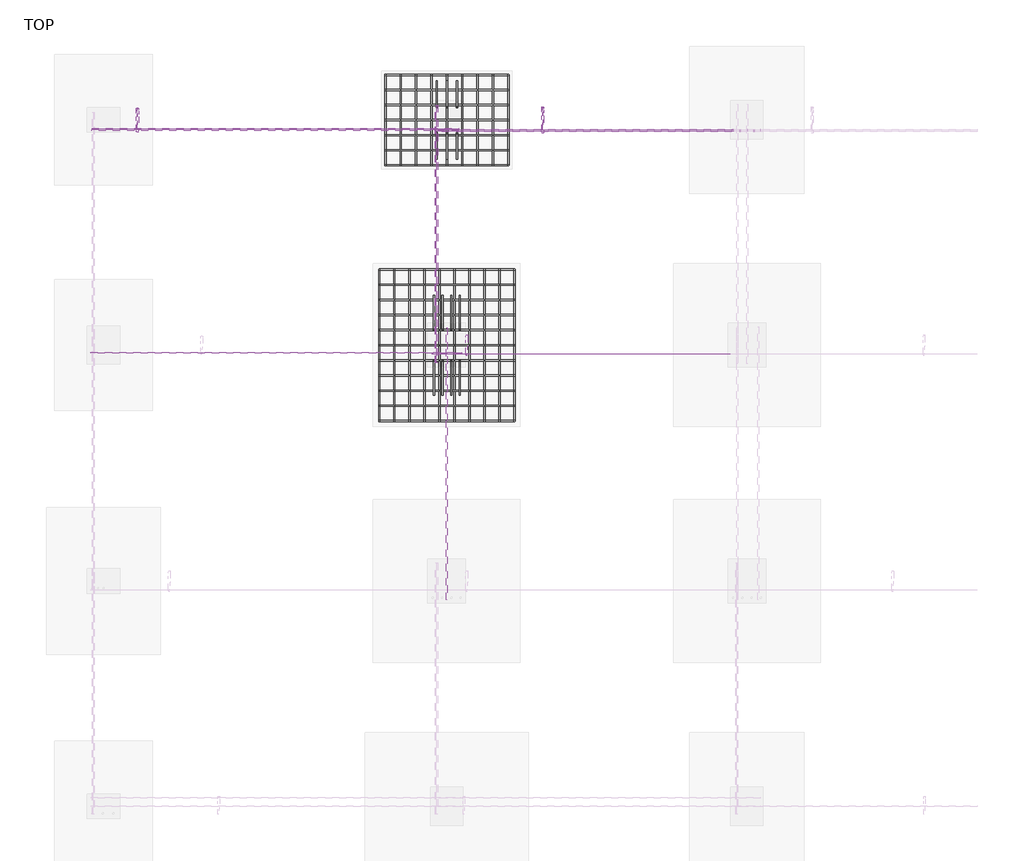
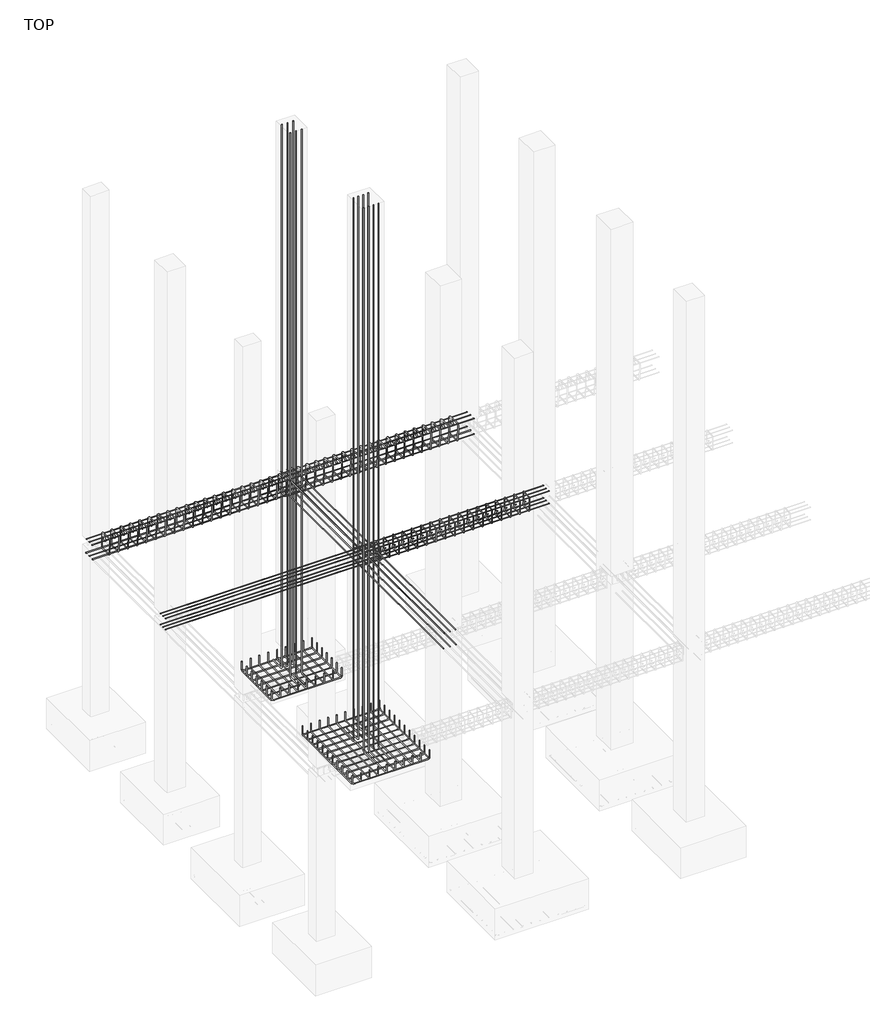
# One storey, part 4 of 8: 23 reinforcing bars.
"""IFC4 building model written with IfcOpenShell, lengths in millimetres."""

from ifc_helpers import new_model, si_unit, point, frame, origin, place, context, project, spatial, polyline, circle_curve, trimmed, segment, composite_curve, source, transform, mapped, element, save
from ifc_brep_helpers import swept_disk

model = new_model("IFC4")

# Units and contexts
model_context = context("Model", 3, world=origin())
ifc_project = project(units=[si_unit("LENGTHUNIT", "METRE", prefix="MILLI")], contexts=[model_context])

# Site, building, storey
site = spatial("IfcSite", under=ifc_project)
building = spatial("IfcBuilding", under=site)
storey = spatial("IfcBuildingStorey", under=building, Name="TOP", Elevation=0.0)

# Reinforcing bars
placement = place(None, origin())
reinforcing_bar_shape = source(origin(), model_context, "Body", "SolidModel", [
    swept_disk(composite_curve([segment(polyline([(-2538.5160601, 7943.1307576, -331.0), (-2538.5160601, 7943.1307576, -467.4)]), True, "CONTINUOUS"), segment(trimmed(circle_curve(frame((-2508.5160601, 7943.1307576, -467.4), z_axis=(0.0, -1.0, 0.0), x_axis=(-30.0, 0.0, 0.0)), 30.0), [point((-2538.5160601, 7943.1307576, -467.4))], [point((-2508.5160601, 7943.1307576, -497.4))], True, "CARTESIAN"), True, "CONTINUOUS"), segment(polyline([(-2508.5160601, 7943.1307576, -497.4), (-1421.3160601, 7943.1307576, -497.4)]), True, "CONTINUOUS"), segment(trimmed(circle_curve(frame((-1421.3160601, 7943.1307576, -467.4), z_axis=(0.0, -1.0, 0.0), x_axis=(0.0, 0.0, -30.0)), 30.0), [point((-1421.3160601, 7943.1307576, -497.4))], [point((-1391.3160601, 7943.1307576, -467.4))], True, "CARTESIAN"), True, "CONTINUOUS"), segment(polyline([(-1391.3160601, 7943.1307576, -467.4), (-1391.3160601, 7943.1307576, -331.0)]), True, "CONTINUOUS")], self_intersect=False), 6.0),
])
element("IfcReinforcingBar", 1, at=placement, inside=storey, context=model_context, shape_type="MappedRepresentation", body=[
    mapped(reinforcing_bar_shape, transform((0.0, 0.0, 0.0), x_axis=(1.0, 0.0, 0.0), y_axis=(0.0, 1.0, 0.0), z_axis=(0.0, 0.0, 1.0))),
    mapped(reinforcing_bar_shape, transform((0.0, -140.4, 0.0), x_axis=(1.0, 0.0, 0.0), y_axis=(0.0, 1.0, 0.0), z_axis=(0.0, 0.0, 1.0))),
    mapped(reinforcing_bar_shape, transform((0.0, -280.8, 0.0), x_axis=(1.0, 0.0, 0.0), y_axis=(0.0, 1.0, 0.0), z_axis=(0.0, 0.0, 1.0))),
    mapped(reinforcing_bar_shape, transform((0.0, -421.2, 0.0), x_axis=(1.0, 0.0, 0.0), y_axis=(0.0, 1.0, 0.0), z_axis=(0.0, 0.0, 1.0))),
    mapped(reinforcing_bar_shape, transform((0.0, -561.6, 0.0), x_axis=(1.0, 0.0, 0.0), y_axis=(0.0, 1.0, 0.0), z_axis=(0.0, 0.0, 1.0))),
    mapped(reinforcing_bar_shape, transform((0.0, -702.0, 0.0), x_axis=(1.0, 0.0, 0.0), y_axis=(0.0, 1.0, 0.0), z_axis=(0.0, 0.0, 1.0))),
    mapped(reinforcing_bar_shape, transform((0.0, -842.4, 0.0), x_axis=(1.0, 0.0, 0.0), y_axis=(0.0, 1.0, 0.0), z_axis=(0.0, 0.0, 1.0))),
])
reinforcing_bar_2_shape = source(origin(), model_context, "Body", "SolidModel", [
    swept_disk(composite_curve([segment(polyline([(-2538.5160601, 7100.7307576, -331.0), (-2538.5160601, 7100.7307576, -467.4)]), True, "CONTINUOUS"), segment(trimmed(circle_curve(frame((-2538.5160601, 7130.7307576, -467.4), z_axis=(1.0, 0.0, 0.0), x_axis=(0.0, -30.0, 0.0)), 30.0), [point((-2538.5160601, 7100.7307576, -467.4))], [point((-2538.5160601, 7130.7307576, -497.4))], True, "CARTESIAN"), True, "CONTINUOUS"), segment(polyline([(-2538.5160601, 7130.7307576, -497.4), (-2538.5160601, 7913.1307576, -497.4)]), True, "CONTINUOUS"), segment(trimmed(circle_curve(frame((-2538.5160601, 7913.1307576, -467.4), z_axis=(1.0, 0.0, 0.0), x_axis=(0.0, 0.0, -30.0)), 30.0), [point((-2538.5160601, 7913.1307576, -497.4))], [point((-2538.5160601, 7943.1307576, -467.4))], True, "CARTESIAN"), True, "CONTINUOUS"), segment(polyline([(-2538.5160601, 7943.1307576, -467.4), (-2538.5160601, 7943.1307576, -331.0)]), True, "CONTINUOUS")], self_intersect=False), 6.0),
])
element("IfcReinforcingBar", 2, at=placement, inside=storey, context=model_context, shape_type="MappedRepresentation", body=[
    mapped(reinforcing_bar_2_shape, transform((0.0, 0.0, 0.0), x_axis=(1.0, 0.0, 0.0), y_axis=(0.0, 1.0, 0.0), z_axis=(0.0, 0.0, 1.0))),
    mapped(reinforcing_bar_2_shape, transform((143.4, 0.0, 0.0), x_axis=(1.0, 0.0, 0.0), y_axis=(0.0, 1.0, 0.0), z_axis=(0.0, 0.0, 1.0))),
    mapped(reinforcing_bar_2_shape, transform((286.8, 0.0, 0.0), x_axis=(1.0, 0.0, 0.0), y_axis=(0.0, 1.0, 0.0), z_axis=(0.0, 0.0, 1.0))),
    mapped(reinforcing_bar_2_shape, transform((430.2, 0.0, 0.0), x_axis=(1.0, 0.0, 0.0), y_axis=(0.0, 1.0, 0.0), z_axis=(0.0, 0.0, 1.0))),
    mapped(reinforcing_bar_2_shape, transform((573.6, 0.0, 0.0), x_axis=(1.0, 0.0, 0.0), y_axis=(0.0, 1.0, 0.0), z_axis=(0.0, 0.0, 1.0))),
    mapped(reinforcing_bar_2_shape, transform((717.0, 0.0, 0.0), x_axis=(1.0, 0.0, 0.0), y_axis=(0.0, 1.0, 0.0), z_axis=(0.0, 0.0, 1.0))),
    mapped(reinforcing_bar_2_shape, transform((860.4, 0.0, 0.0), x_axis=(1.0, 0.0, 0.0), y_axis=(0.0, 1.0, 0.0), z_axis=(0.0, 0.0, 1.0))),
    mapped(reinforcing_bar_2_shape, transform((1003.8, 0.0, 0.0), x_axis=(1.0, 0.0, 0.0), y_axis=(0.0, 1.0, 0.0), z_axis=(0.0, 0.0, 1.0))),
    mapped(reinforcing_bar_2_shape, transform((1147.2, 0.0, 0.0), x_axis=(1.0, 0.0, 0.0), y_axis=(0.0, 1.0, 0.0), z_axis=(0.0, 0.0, 1.0))),
])
reinforcing_bar_3_shape = source(origin(), model_context, "Body", "SolidModel", [
    swept_disk(composite_curve([segment(polyline([(-2059.3160601, 7641.7815576, 8958.464), (-2059.3160601, 7641.7815576, -409.536)]), True, "CONTINUOUS"), segment(trimmed(circle_curve(frame((-2059.3160601, 7671.7815576, -409.536), z_axis=(1.0, 0.0, 0.0), x_axis=(0.0, -30.0, 0.0)), 30.0), [point((-2059.3160601, 7641.7815576, -409.536))], [point((-2059.3160601, 7671.7815576, -439.536))], True, "CARTESIAN"), True, "CONTINUOUS"), segment(polyline([(-2059.3160601, 7671.7815576, -439.536), (-2059.3160601, 7888.3815576, -439.536)]), True, "CONTINUOUS")], self_intersect=False), 6.0),
])
element("IfcReinforcingBar", 3, at=placement, inside=storey, context=model_context, shape_type="MappedRepresentation", body=[
    mapped(reinforcing_bar_3_shape, transform((0.0, 0.0, 0.0), x_axis=(1.0, 0.0, 0.0), y_axis=(0.0, 1.0, 0.0), z_axis=(0.0, 0.0, 1.0))),
    mapped(reinforcing_bar_3_shape, transform((94.4, 0.0, 0.0), x_axis=(1.0, 0.0, 0.0), y_axis=(0.0, 1.0, 0.0), z_axis=(0.0, 0.0, 1.0))),
    mapped(reinforcing_bar_3_shape, transform((188.8, 0.0, 0.0), x_axis=(1.0, 0.0, 0.0), y_axis=(0.0, 1.0, 0.0), z_axis=(0.0, 0.0, 1.0))),
])
reinforcing_bar_4_shape = source(origin(), model_context, "Body", "SolidModel", [
    swept_disk(composite_curve([segment(polyline([(-1870.5160601, 7402.0799576, 8958.464), (-1870.5160601, 7402.0799576, -415.886)]), True, "CONTINUOUS"), segment(trimmed(circle_curve(frame((-1870.5160601, 7372.0799576, -415.886), z_axis=(-1.0, 0.0, 0.0), x_axis=(0.0, 30.0, 0.0)), 30.0), [point((-1870.5160601, 7402.0799576, -415.886))], [point((-1870.5160601, 7372.0799576, -445.886))], True, "CARTESIAN"), True, "CONTINUOUS"), segment(polyline([(-1870.5160601, 7372.0799576, -445.886), (-1870.5160601, 7155.4799576, -445.886)]), True, "CONTINUOUS")], self_intersect=False), 6.0),
])
element("IfcReinforcingBar", 4, at=placement, inside=storey, context=model_context, shape_type="MappedRepresentation", body=[
    mapped(reinforcing_bar_4_shape, transform((0.0, 0.0, 0.0), x_axis=(1.0, 0.0, 0.0), y_axis=(0.0, 1.0, 0.0), z_axis=(0.0, 0.0, 1.0))),
    mapped(reinforcing_bar_4_shape, transform((-94.4, 0.0, 0.0), x_axis=(1.0, 0.0, 0.0), y_axis=(0.0, 1.0, 0.0), z_axis=(0.0, 0.0, 1.0))),
    mapped(reinforcing_bar_4_shape, transform((-188.8, 0.0, 0.0), x_axis=(1.0, 0.0, 0.0), y_axis=(0.0, 1.0, 0.0), z_axis=(0.0, 0.0, 1.0))),
])
reinforcing_bar_5_shape = source(origin(), model_context, "Body", "SolidModel", [
    swept_disk(composite_curve([segment(polyline([(-2594.7160601, 6127.9307576, -331.0), (-2594.7160601, 6127.9307576, -447.4)]), True, "CONTINUOUS"), segment(trimmed(circle_curve(frame((-2564.7160601, 6127.9307576, -447.4), z_axis=(0.0, -1.0, 0.0), x_axis=(-30.0, 0.0, 0.0)), 30.0), [point((-2594.7160601, 6127.9307576, -447.4))], [point((-2564.7160601, 6127.9307576, -477.4))], True, "CARTESIAN"), True, "CONTINUOUS"), segment(polyline([(-2564.7160601, 6127.9307576, -477.4), (-1365.1160601, 6127.9307576, -477.4)]), True, "CONTINUOUS"), segment(trimmed(circle_curve(frame((-1365.1160601, 6127.9307576, -447.4), z_axis=(0.0, -1.0, 0.0), x_axis=(0.0, 0.0, -30.0)), 30.0), [point((-1365.1160601, 6127.9307576, -477.4))], [point((-1335.1160601, 6127.9307576, -447.4))], True, "CARTESIAN"), True, "CONTINUOUS"), segment(polyline([(-1335.1160601, 6127.9307576, -447.4), (-1335.1160601, 6127.9307576, -331.0)]), True, "CONTINUOUS")], self_intersect=False), 6.0),
])
element("IfcReinforcingBar", 5, at=placement, inside=storey, context=model_context, shape_type="MappedRepresentation", body=[
    mapped(reinforcing_bar_5_shape, transform((0.0, 0.0, 0.0), x_axis=(1.0, 0.0, 0.0), y_axis=(0.0, 1.0, 0.0), z_axis=(0.0, 0.0, 1.0))),
    mapped(reinforcing_bar_5_shape, transform((0.0, -141.2, 0.0), x_axis=(1.0, 0.0, 0.0), y_axis=(0.0, 1.0, 0.0), z_axis=(0.0, 0.0, 1.0))),
    mapped(reinforcing_bar_5_shape, transform((0.0, -282.4, 0.0), x_axis=(1.0, 0.0, 0.0), y_axis=(0.0, 1.0, 0.0), z_axis=(0.0, 0.0, 1.0))),
    mapped(reinforcing_bar_5_shape, transform((0.0, -423.6, 0.0), x_axis=(1.0, 0.0, 0.0), y_axis=(0.0, 1.0, 0.0), z_axis=(0.0, 0.0, 1.0))),
    mapped(reinforcing_bar_5_shape, transform((0.0, -564.8, 0.0), x_axis=(1.0, 0.0, 0.0), y_axis=(0.0, 1.0, 0.0), z_axis=(0.0, 0.0, 1.0))),
    mapped(reinforcing_bar_5_shape, transform((0.0, -706.0, 0.0), x_axis=(1.0, 0.0, 0.0), y_axis=(0.0, 1.0, 0.0), z_axis=(0.0, 0.0, 1.0))),
    mapped(reinforcing_bar_5_shape, transform((0.0, -847.2, 0.0), x_axis=(1.0, 0.0, 0.0), y_axis=(0.0, 1.0, 0.0), z_axis=(0.0, 0.0, 1.0))),
    mapped(reinforcing_bar_5_shape, transform((0.0, -988.4, 0.0), x_axis=(1.0, 0.0, 0.0), y_axis=(0.0, 1.0, 0.0), z_axis=(0.0, 0.0, 1.0))),
    mapped(reinforcing_bar_5_shape, transform((0.0, -1129.6, 0.0), x_axis=(1.0, 0.0, 0.0), y_axis=(0.0, 1.0, 0.0), z_axis=(0.0, 0.0, 1.0))),
    mapped(reinforcing_bar_5_shape, transform((0.0, -1270.8, 0.0), x_axis=(1.0, 0.0, 0.0), y_axis=(0.0, 1.0, 0.0), z_axis=(0.0, 0.0, 1.0))),
    mapped(reinforcing_bar_5_shape, transform((0.0, -1412.0, 0.0), x_axis=(1.0, 0.0, 0.0), y_axis=(0.0, 1.0, 0.0), z_axis=(0.0, 0.0, 1.0))),
])
reinforcing_bar_6_shape = source(origin(), model_context, "Body", "SolidModel", [
    swept_disk(composite_curve([segment(polyline([(-2594.7160601, 4715.9307576, -331.0), (-2594.7160601, 4715.9307576, -447.4)]), True, "CONTINUOUS"), segment(trimmed(circle_curve(frame((-2594.7160601, 4745.9307576, -447.4), z_axis=(1.0, 0.0, 0.0), x_axis=(0.0, -30.0, 0.0)), 30.0), [point((-2594.7160601, 4715.9307576, -447.4))], [point((-2594.7160601, 4745.9307576, -477.4))], True, "CARTESIAN"), True, "CONTINUOUS"), segment(polyline([(-2594.7160601, 4745.9307576, -477.4), (-2594.7160601, 6097.9307576, -477.4)]), True, "CONTINUOUS"), segment(trimmed(circle_curve(frame((-2594.7160601, 6097.9307576, -447.4), z_axis=(1.0, 0.0, 0.0), x_axis=(0.0, 0.0, -30.0)), 30.0), [point((-2594.7160601, 6097.9307576, -477.4))], [point((-2594.7160601, 6127.9307576, -447.4))], True, "CARTESIAN"), True, "CONTINUOUS"), segment(polyline([(-2594.7160601, 6127.9307576, -447.4), (-2594.7160601, 6127.9307576, -331.0)]), True, "CONTINUOUS")], self_intersect=False), 6.0),
])
element("IfcReinforcingBar", 6, at=placement, inside=storey, context=model_context, shape_type="MappedRepresentation", body=[
    mapped(reinforcing_bar_6_shape, transform((0.0, 0.0, 0.0), x_axis=(1.0, 0.0, 0.0), y_axis=(0.0, 1.0, 0.0), z_axis=(0.0, 0.0, 1.0))),
    mapped(reinforcing_bar_6_shape, transform((139.9555556, 0.0, 0.0), x_axis=(1.0, 0.0, 0.0), y_axis=(0.0, 1.0, 0.0), z_axis=(0.0, 0.0, 1.0))),
    mapped(reinforcing_bar_6_shape, transform((279.9111111, 0.0, 0.0), x_axis=(1.0, 0.0, 0.0), y_axis=(0.0, 1.0, 0.0), z_axis=(0.0, 0.0, 1.0))),
    mapped(reinforcing_bar_6_shape, transform((419.8666667, 0.0, 0.0), x_axis=(1.0, 0.0, 0.0), y_axis=(0.0, 1.0, 0.0), z_axis=(0.0, 0.0, 1.0))),
    mapped(reinforcing_bar_6_shape, transform((559.8222222, 0.0, 0.0), x_axis=(1.0, 0.0, 0.0), y_axis=(0.0, 1.0, 0.0), z_axis=(0.0, 0.0, 1.0))),
    mapped(reinforcing_bar_6_shape, transform((699.7777778, 0.0, 0.0), x_axis=(1.0, 0.0, 0.0), y_axis=(0.0, 1.0, 0.0), z_axis=(0.0, 0.0, 1.0))),
    mapped(reinforcing_bar_6_shape, transform((839.7333333, 0.0, 0.0), x_axis=(1.0, 0.0, 0.0), y_axis=(0.0, 1.0, 0.0), z_axis=(0.0, 0.0, 1.0))),
    mapped(reinforcing_bar_6_shape, transform((979.6888889, 0.0, 0.0), x_axis=(1.0, 0.0, 0.0), y_axis=(0.0, 1.0, 0.0), z_axis=(0.0, 0.0, 1.0))),
    mapped(reinforcing_bar_6_shape, transform((1119.6444444, 0.0, 0.0), x_axis=(1.0, 0.0, 0.0), y_axis=(0.0, 1.0, 0.0), z_axis=(0.0, 0.0, 1.0))),
    mapped(reinforcing_bar_6_shape, transform((1259.6, 0.0, 0.0), x_axis=(1.0, 0.0, 0.0), y_axis=(0.0, 1.0, 0.0), z_axis=(0.0, 0.0, 1.0))),
])
reinforcing_bar_7_shape = source(origin(), model_context, "Body", "SolidModel", [
    swept_disk(composite_curve([segment(polyline([(-2084.7668601, 5567.0799576, 8958.464), (-2084.7668601, 5567.0799576, -403.186)]), True, "CONTINUOUS"), segment(trimmed(circle_curve(frame((-2084.7668601, 5597.0799576, -403.186), z_axis=(1.0, 0.0, 0.0), x_axis=(0.0, -30.0, 0.0)), 30.0), [point((-2084.7668601, 5567.0799576, -403.186))], [point((-2084.7668601, 5597.0799576, -433.186))], True, "CARTESIAN"), True, "CONTINUOUS"), segment(polyline([(-2084.7668601, 5597.0799576, -433.186), (-2084.7668601, 5889.8799576, -433.186)]), True, "CONTINUOUS")], self_intersect=False), 6.0),
])
element("IfcReinforcingBar", 7, at=placement, inside=storey, context=model_context, shape_type="MappedRepresentation", body=[
    mapped(reinforcing_bar_7_shape, transform((0.0, 0.0, 0.0), x_axis=(1.0, 0.0, 0.0), y_axis=(0.0, 1.0, 0.0), z_axis=(0.0, 0.0, 1.0))),
    mapped(reinforcing_bar_7_shape, transform((79.9005333, 0.0, 0.0), x_axis=(1.0, 0.0, 0.0), y_axis=(0.0, 1.0, 0.0), z_axis=(0.0, 0.0, 1.0))),
    mapped(reinforcing_bar_7_shape, transform((159.8010667, 0.0, 0.0), x_axis=(1.0, 0.0, 0.0), y_axis=(0.0, 1.0, 0.0), z_axis=(0.0, 0.0, 1.0))),
    mapped(reinforcing_bar_7_shape, transform((239.7016, 0.0, 0.0), x_axis=(1.0, 0.0, 0.0), y_axis=(0.0, 1.0, 0.0), z_axis=(0.0, 0.0, 1.0))),
])
reinforcing_bar_8_shape = source(origin(), model_context, "Body", "SolidModel", [
    swept_disk(composite_curve([segment(polyline([(-1845.0652601, 5276.7815576, 8958.464), (-1845.0652601, 5276.7815576, -409.536)]), True, "CONTINUOUS"), segment(trimmed(circle_curve(frame((-1845.0652601, 5246.7815576, -409.536), z_axis=(-1.0, 0.0, 0.0), x_axis=(0.0, 30.0, 0.0)), 30.0), [point((-1845.0652601, 5276.7815576, -409.536))], [point((-1845.0652601, 5246.7815576, -439.536))], True, "CARTESIAN"), True, "CONTINUOUS"), segment(polyline([(-1845.0652601, 5246.7815576, -439.536), (-1845.0652601, 4953.9815576, -439.536)]), True, "CONTINUOUS")], self_intersect=False), 6.0),
])
element("IfcReinforcingBar", 8, at=placement, inside=storey, context=model_context, shape_type="MappedRepresentation", body=[
    mapped(reinforcing_bar_8_shape, transform((0.0, 0.0, 0.0), x_axis=(1.0, 0.0, 0.0), y_axis=(0.0, 1.0, 0.0), z_axis=(0.0, 0.0, 1.0))),
    mapped(reinforcing_bar_8_shape, transform((-79.9005333, 0.0, 0.0), x_axis=(1.0, 0.0, 0.0), y_axis=(0.0, 1.0, 0.0), z_axis=(0.0, 0.0, 1.0))),
    mapped(reinforcing_bar_8_shape, transform((-159.8010667, 0.0, 0.0), x_axis=(1.0, 0.0, 0.0), y_axis=(0.0, 1.0, 0.0), z_axis=(0.0, 0.0, 1.0))),
    mapped(reinforcing_bar_8_shape, transform((-239.7016, 0.0, 0.0), x_axis=(1.0, 0.0, 0.0), y_axis=(0.0, 1.0, 0.0), z_axis=(0.0, 0.0, 1.0))),
])
reinforcing_bar_9_shape = source(origin(), model_context, "Body", "SolidModel", [
    swept_disk(composite_curve([segment(polyline([(-2122.3160601, 7515.94241, 2876.9669914), (-2122.3160601, 7586.6530881, 2947.6776695)]), True, "CONTINUOUS"), segment(trimmed(circle_curve(frame((-2122.3160601, 7604.3307576, 2930.0), z_axis=(-1.0, 0.0, 0.0), x_axis=(0.0, -17.677669499999865, 17.677669499999865)), 25.0), [point((-2122.3160601, 7586.6530881, 2947.6776695))], [point((-2122.3160601, 7629.3307576, 2930.0))], True, "CARTESIAN"), True, "CONTINUOUS"), segment(polyline([(-2122.3160601, 7629.3307576, 2930.0), (-2122.3160601, 7629.3307576, 2714.2984)]), True, "CONTINUOUS"), segment(trimmed(circle_curve(frame((-2122.3160601, 7604.3307576, 2714.2984), z_axis=(-1.0, 0.0, 0.0), x_axis=(0.0, 25.0, 0.0)), 25.0), [point((-2122.3160601, 7629.3307576, 2714.2984))], [point((-2122.3160601, 7604.3307576, 2689.2984))], True, "CARTESIAN"), True, "CONTINUOUS"), segment(polyline([(-2122.3160601, 7604.3307576, 2689.2984), (-2122.3160601, 7439.5307576, 2689.2984)]), True, "CONTINUOUS"), segment(trimmed(circle_curve(frame((-2121.3758206, 7439.5307576, 2714.2807127), z_axis=(-0.9992925095435161, 0.0, 0.03760957817128376), x_axis=(-0.9402394999997341, 0.0, -24.982312699999966)), 25.0), [point((-2122.3160601, 7439.5307576, 2689.2984))], [point((-2121.3758206, 7414.5307576, 2714.2807127))], True, "CARTESIAN"), True, "CONTINUOUS"), segment(polyline([(-2121.3758206, 7414.5307576, 2714.2807127), (-2113.2562995, 7414.5307576, 2930.0176873)]), True, "CONTINUOUS"), segment(trimmed(circle_curve(frame((-2113.2562995, 7439.5307576, 2930.0176873), z_axis=(-0.9992925095435161, 0.0, 0.03760957817128376), x_axis=(0.0, -25.0, 0.0)), 25.0), [point((-2113.2562995, 7414.5307576, 2930.0176873))], [point((-2112.3160601, 7439.5307576, 2955.0))], True, "CARTESIAN"), True, "CONTINUOUS"), segment(polyline([(-2112.3160601, 7439.5307576, 2955.0), (-2112.3160601, 7604.3307576, 2955.0)]), True, "CONTINUOUS"), segment(trimmed(circle_curve(frame((-2112.3160601, 7604.3307576, 2930.0), z_axis=(-1.0, 0.0, 0.0), x_axis=(0.0, 0.0, 25.0)), 25.0), [point((-2112.3160601, 7604.3307576, 2955.0))], [point((-2112.3160601, 7622.0084271, 2912.3223305))], True, "CARTESIAN"), True, "CONTINUOUS"), segment(polyline([(-2112.3160601, 7622.0084271, 2912.3223305), (-2112.3160601, 7551.297749, 2841.6116524)]), True, "CONTINUOUS")], self_intersect=False), 5.0),
])
element("IfcReinforcingBar", 9, at=placement, inside=storey, context=model_context, shape_type="MappedRepresentation", body=[
    mapped(reinforcing_bar_9_shape, transform((0.0, 0.0, 0.0), x_axis=(1.0, 0.0, 0.0), y_axis=(0.0, 1.0, 0.0), z_axis=(0.0, 0.0, 1.0))),
    mapped(reinforcing_bar_9_shape, transform((-151.8526316, 0.0, 0.0), x_axis=(1.0, 0.0, 0.0), y_axis=(0.0, 1.0, 0.0), z_axis=(0.0, 0.0, 1.0))),
    mapped(reinforcing_bar_9_shape, transform((-303.7052632, 0.0, 0.0), x_axis=(1.0, 0.0, 0.0), y_axis=(0.0, 1.0, 0.0), z_axis=(0.0, 0.0, 1.0))),
    mapped(reinforcing_bar_9_shape, transform((-455.5578947, 0.0, 0.0), x_axis=(1.0, 0.0, 0.0), y_axis=(0.0, 1.0, 0.0), z_axis=(0.0, 0.0, 1.0))),
    mapped(reinforcing_bar_9_shape, transform((-607.4105263, 0.0, 0.0), x_axis=(1.0, 0.0, 0.0), y_axis=(0.0, 1.0, 0.0), z_axis=(0.0, 0.0, 1.0))),
    mapped(reinforcing_bar_9_shape, transform((-759.2631579, 0.0, 0.0), x_axis=(1.0, 0.0, 0.0), y_axis=(0.0, 1.0, 0.0), z_axis=(0.0, 0.0, 1.0))),
    mapped(reinforcing_bar_9_shape, transform((-911.1157895, 0.0, 0.0), x_axis=(1.0, 0.0, 0.0), y_axis=(0.0, 1.0, 0.0), z_axis=(0.0, 0.0, 1.0))),
    mapped(reinforcing_bar_9_shape, transform((-1062.9684211, 0.0, 0.0), x_axis=(1.0, 0.0, 0.0), y_axis=(0.0, 1.0, 0.0), z_axis=(0.0, 0.0, 1.0))),
    mapped(reinforcing_bar_9_shape, transform((-1214.8210526, 0.0, 0.0), x_axis=(1.0, 0.0, 0.0), y_axis=(0.0, 1.0, 0.0), z_axis=(0.0, 0.0, 1.0))),
    mapped(reinforcing_bar_9_shape, transform((-1366.6736842, 0.0, 0.0), x_axis=(1.0, 0.0, 0.0), y_axis=(0.0, 1.0, 0.0), z_axis=(0.0, 0.0, 1.0))),
    mapped(reinforcing_bar_9_shape, transform((-1518.5263158, 0.0, 0.0), x_axis=(1.0, 0.0, 0.0), y_axis=(0.0, 1.0, 0.0), z_axis=(0.0, 0.0, 1.0))),
    mapped(reinforcing_bar_9_shape, transform((-1670.3789474, 0.0, 0.0), x_axis=(1.0, 0.0, 0.0), y_axis=(0.0, 1.0, 0.0), z_axis=(0.0, 0.0, 1.0))),
    mapped(reinforcing_bar_9_shape, transform((-1822.2315789, 0.0, 0.0), x_axis=(1.0, 0.0, 0.0), y_axis=(0.0, 1.0, 0.0), z_axis=(0.0, 0.0, 1.0))),
    mapped(reinforcing_bar_9_shape, transform((-1974.0842105, 0.0, 0.0), x_axis=(1.0, 0.0, 0.0), y_axis=(0.0, 1.0, 0.0), z_axis=(0.0, 0.0, 1.0))),
    mapped(reinforcing_bar_9_shape, transform((-2125.9368421, 0.0, 0.0), x_axis=(1.0, 0.0, 0.0), y_axis=(0.0, 1.0, 0.0), z_axis=(0.0, 0.0, 1.0))),
    mapped(reinforcing_bar_9_shape, transform((-2277.7894737, 0.0, 0.0), x_axis=(1.0, 0.0, 0.0), y_axis=(0.0, 1.0, 0.0), z_axis=(0.0, 0.0, 1.0))),
    mapped(reinforcing_bar_9_shape, transform((-2429.6421053, 0.0, 0.0), x_axis=(1.0, 0.0, 0.0), y_axis=(0.0, 1.0, 0.0), z_axis=(0.0, 0.0, 1.0))),
    mapped(reinforcing_bar_9_shape, transform((-2581.4947368, 0.0, 0.0), x_axis=(1.0, 0.0, 0.0), y_axis=(0.0, 1.0, 0.0), z_axis=(0.0, 0.0, 1.0))),
    mapped(reinforcing_bar_9_shape, transform((-2733.3473684, 0.0, 0.0), x_axis=(1.0, 0.0, 0.0), y_axis=(0.0, 1.0, 0.0), z_axis=(0.0, 0.0, 1.0))),
    mapped(reinforcing_bar_9_shape, transform((-2885.2, 0.0, 0.0), x_axis=(1.0, 0.0, 0.0), y_axis=(0.0, 1.0, 0.0), z_axis=(0.0, 0.0, 1.0))),
])
reinforcing_bar_10_shape = source(origin(), model_context, "Body", "SolidModel", [
    swept_disk(composite_curve([segment(polyline([(-1852.5160601, 7614.9373593, 2703.6917983), (-5277.3160601, 7614.9373593, 2703.6917983)]), True, "CONTINUOUS")], self_intersect=False), 5.0),
])
element("IfcReinforcingBar", 10, at=placement, inside=storey, context=model_context, shape_type="MappedRepresentation", body=[
    mapped(reinforcing_bar_10_shape, transform((0.0, 0.0, 0.0), x_axis=(1.0, 0.0, 0.0), y_axis=(0.0, 1.0, 0.0), z_axis=(0.0, 0.0, 1.0))),
    mapped(reinforcing_bar_10_shape, transform((0.0, -93.0066017, 0.0), x_axis=(1.0, 0.0, 0.0), y_axis=(0.0, 1.0, 0.0), z_axis=(0.0, 0.0, 1.0))),
    mapped(reinforcing_bar_10_shape, transform((0.0, -186.0132034, 0.0), x_axis=(1.0, 0.0, 0.0), y_axis=(0.0, 1.0, 0.0), z_axis=(0.0, 0.0, 1.0))),
])
reinforcing_bar_11_shape = source(origin(), model_context, "Body", "SolidModel", [
    swept_disk(composite_curve([segment(polyline([(-5277.3160601, 7604.3307576, 2945.0), (-1852.5160601, 7604.3307576, 2945.0)]), True, "CONTINUOUS")], self_intersect=False), 5.0),
])
element("IfcReinforcingBar", 11, at=placement, inside=storey, context=model_context, shape_type="MappedRepresentation", body=[
    mapped(reinforcing_bar_11_shape, transform((0.0, 0.0, 0.0), x_axis=(1.0, 0.0, 0.0), y_axis=(0.0, 1.0, 0.0), z_axis=(0.0, 0.0, 1.0))),
    mapped(reinforcing_bar_11_shape, transform((0.0, -82.4, 0.0), x_axis=(1.0, 0.0, 0.0), y_axis=(0.0, 1.0, 0.0), z_axis=(0.0, 0.0, 1.0))),
    mapped(reinforcing_bar_11_shape, transform((0.0, -164.8, 0.0), x_axis=(1.0, 0.0, 0.0), y_axis=(0.0, 1.0, 0.0), z_axis=(0.0, 0.0, 1.0))),
])
reinforcing_bar_12_shape = source(origin(), model_context, "Body", "SolidModel", [
    swept_disk(composite_curve([segment(polyline([(677.6839399, 7525.94241, 2886.9669914), (677.6839399, 7596.6530881, 2957.6776695)]), True, "CONTINUOUS"), segment(trimmed(circle_curve(frame((677.6839399, 7614.3307576, 2940.0), z_axis=(-1.0, 0.0, 0.0), x_axis=(0.0, -17.677669499999865, 17.677669499999865)), 25.0), [point((677.6839399, 7596.6530881, 2957.6776695))], [point((677.6839399, 7639.3307576, 2940.0))], True, "CARTESIAN"), True, "CONTINUOUS"), segment(polyline([(677.6839399, 7639.3307576, 2940.0), (677.6839399, 7639.3307576, 2704.2984)]), True, "CONTINUOUS"), segment(trimmed(circle_curve(frame((677.6839399, 7614.3307576, 2704.2984), z_axis=(-1.0, 0.0, 0.0), x_axis=(0.0, 25.0, 0.0)), 25.0), [point((677.6839399, 7639.3307576, 2704.2984))], [point((677.6839399, 7614.3307576, 2679.2984))], True, "CARTESIAN"), True, "CONTINUOUS"), segment(polyline([(677.6839399, 7614.3307576, 2679.2984), (677.6839399, 7429.5307576, 2679.2984)]), True, "CONTINUOUS"), segment(trimmed(circle_curve(frame((678.5584433, 7429.5307576, 2704.2831002), z_axis=(-0.9993880078667093, 0.0, 0.034980133393257534), x_axis=(-0.8745033999999805, 0.0, -24.98470019999968)), 25.0), [point((677.6839399, 7429.5307576, 2679.2984))], [point((678.5584433, 7404.5307576, 2704.2831002))], True, "CARTESIAN"), True, "CONTINUOUS"), segment(polyline([(678.5584433, 7404.5307576, 2704.2831002), (686.8094366, 7404.5307576, 2940.0152998)]), True, "CONTINUOUS"), segment(trimmed(circle_curve(frame((686.8094366, 7429.5307576, 2940.0152998), z_axis=(-0.9993880078667093, 0.0, 0.034980133393257534), x_axis=(0.0, -25.0, 0.0)), 25.0), [point((686.8094366, 7404.5307576, 2940.0152998))], [point((687.6839399, 7429.5307576, 2965.0))], True, "CARTESIAN"), True, "CONTINUOUS"), segment(polyline([(687.6839399, 7429.5307576, 2965.0), (687.6839399, 7614.3307576, 2965.0)]), True, "CONTINUOUS"), segment(trimmed(circle_curve(frame((687.6839399, 7614.3307576, 2940.0), z_axis=(-1.0, 0.0, 0.0), x_axis=(0.0, 0.0, 25.0)), 25.0), [point((687.6839399, 7614.3307576, 2965.0))], [point((687.6839399, 7632.0084271, 2922.3223305))], True, "CARTESIAN"), True, "CONTINUOUS"), segment(polyline([(687.6839399, 7632.0084271, 2922.3223305), (687.6839399, 7561.297749, 2851.6116524)]), True, "CONTINUOUS")], self_intersect=False), 5.0),
])
element("IfcReinforcingBar", 12, at=placement, inside=storey, context=model_context, shape_type="MappedRepresentation", body=[
    mapped(reinforcing_bar_12_shape, transform((0.0, 0.0, 0.0), x_axis=(1.0, 0.0, 0.0), y_axis=(0.0, 1.0, 0.0), z_axis=(0.0, 0.0, 1.0))),
    mapped(reinforcing_bar_12_shape, transform((-146.1882353, 0.0, 0.0), x_axis=(1.0, 0.0, 0.0), y_axis=(0.0, 1.0, 0.0), z_axis=(0.0, 0.0, 1.0))),
    mapped(reinforcing_bar_12_shape, transform((-292.3764706, 0.0, 0.0), x_axis=(1.0, 0.0, 0.0), y_axis=(0.0, 1.0, 0.0), z_axis=(0.0, 0.0, 1.0))),
    mapped(reinforcing_bar_12_shape, transform((-438.5647059, 0.0, 0.0), x_axis=(1.0, 0.0, 0.0), y_axis=(0.0, 1.0, 0.0), z_axis=(0.0, 0.0, 1.0))),
    mapped(reinforcing_bar_12_shape, transform((-584.7529412, 0.0, 0.0), x_axis=(1.0, 0.0, 0.0), y_axis=(0.0, 1.0, 0.0), z_axis=(0.0, 0.0, 1.0))),
    mapped(reinforcing_bar_12_shape, transform((-730.9411765, 0.0, 0.0), x_axis=(1.0, 0.0, 0.0), y_axis=(0.0, 1.0, 0.0), z_axis=(0.0, 0.0, 1.0))),
    mapped(reinforcing_bar_12_shape, transform((-877.1294118, 0.0, 0.0), x_axis=(1.0, 0.0, 0.0), y_axis=(0.0, 1.0, 0.0), z_axis=(0.0, 0.0, 1.0))),
    mapped(reinforcing_bar_12_shape, transform((-1023.3176471, 0.0, 0.0), x_axis=(1.0, 0.0, 0.0), y_axis=(0.0, 1.0, 0.0), z_axis=(0.0, 0.0, 1.0))),
    mapped(reinforcing_bar_12_shape, transform((-1169.5058824, 0.0, 0.0), x_axis=(1.0, 0.0, 0.0), y_axis=(0.0, 1.0, 0.0), z_axis=(0.0, 0.0, 1.0))),
    mapped(reinforcing_bar_12_shape, transform((-1315.6941176, 0.0, 0.0), x_axis=(1.0, 0.0, 0.0), y_axis=(0.0, 1.0, 0.0), z_axis=(0.0, 0.0, 1.0))),
    mapped(reinforcing_bar_12_shape, transform((-1461.8823529, 0.0, 0.0), x_axis=(1.0, 0.0, 0.0), y_axis=(0.0, 1.0, 0.0), z_axis=(0.0, 0.0, 1.0))),
    mapped(reinforcing_bar_12_shape, transform((-1608.0705882, 0.0, 0.0), x_axis=(1.0, 0.0, 0.0), y_axis=(0.0, 1.0, 0.0), z_axis=(0.0, 0.0, 1.0))),
    mapped(reinforcing_bar_12_shape, transform((-1754.2588235, 0.0, 0.0), x_axis=(1.0, 0.0, 0.0), y_axis=(0.0, 1.0, 0.0), z_axis=(0.0, 0.0, 1.0))),
    mapped(reinforcing_bar_12_shape, transform((-1900.4470588, 0.0, 0.0), x_axis=(1.0, 0.0, 0.0), y_axis=(0.0, 1.0, 0.0), z_axis=(0.0, 0.0, 1.0))),
    mapped(reinforcing_bar_12_shape, transform((-2046.6352941, 0.0, 0.0), x_axis=(1.0, 0.0, 0.0), y_axis=(0.0, 1.0, 0.0), z_axis=(0.0, 0.0, 1.0))),
    mapped(reinforcing_bar_12_shape, transform((-2192.8235294, 0.0, 0.0), x_axis=(1.0, 0.0, 0.0), y_axis=(0.0, 1.0, 0.0), z_axis=(0.0, 0.0, 1.0))),
    mapped(reinforcing_bar_12_shape, transform((-2339.0117647, 0.0, 0.0), x_axis=(1.0, 0.0, 0.0), y_axis=(0.0, 1.0, 0.0), z_axis=(0.0, 0.0, 1.0))),
    mapped(reinforcing_bar_12_shape, transform((-2485.2, 0.0, 0.0), x_axis=(1.0, 0.0, 0.0), y_axis=(0.0, 1.0, 0.0), z_axis=(0.0, 0.0, 1.0))),
])
reinforcing_bar_13_shape = source(origin(), model_context, "Body", "SolidModel", [
    swept_disk(composite_curve([segment(polyline([(957.4839399, 7624.9373593, 2693.6917983), (-2077.3160601, 7624.9373593, 2693.6917983)]), True, "CONTINUOUS")], self_intersect=False), 5.0),
])
element("IfcReinforcingBar", 13, at=placement, inside=storey, context=model_context, shape_type="MappedRepresentation", body=[
    mapped(reinforcing_bar_13_shape, transform((0.0, 0.0, 0.0), x_axis=(1.0, 0.0, 0.0), y_axis=(0.0, 1.0, 0.0), z_axis=(0.0, 0.0, 1.0))),
    mapped(reinforcing_bar_13_shape, transform((0.0, -103.0066017, 0.0), x_axis=(1.0, 0.0, 0.0), y_axis=(0.0, 1.0, 0.0), z_axis=(0.0, 0.0, 1.0))),
    mapped(reinforcing_bar_13_shape, transform((0.0, -206.0132034, 0.0), x_axis=(1.0, 0.0, 0.0), y_axis=(0.0, 1.0, 0.0), z_axis=(0.0, 0.0, 1.0))),
])
reinforcing_bar_14_shape = source(origin(), model_context, "Body", "SolidModel", [
    swept_disk(composite_curve([segment(polyline([(-2077.3160601, 7614.3307576, 2955.0), (957.4839399, 7614.3307576, 2955.0)]), True, "CONTINUOUS")], self_intersect=False), 5.0),
])
element("IfcReinforcingBar", 14, at=placement, inside=storey, context=model_context, shape_type="MappedRepresentation", body=[
    mapped(reinforcing_bar_14_shape, transform((0.0, 0.0, 0.0), x_axis=(1.0, 0.0, 0.0), y_axis=(0.0, 1.0, 0.0), z_axis=(0.0, 0.0, 1.0))),
    mapped(reinforcing_bar_14_shape, transform((0.0, -92.4, 0.0), x_axis=(1.0, 0.0, 0.0), y_axis=(0.0, 1.0, 0.0), z_axis=(0.0, 0.0, 1.0))),
    mapped(reinforcing_bar_14_shape, transform((0.0, -184.8, 0.0), x_axis=(1.0, 0.0, 0.0), y_axis=(0.0, 1.0, 0.0), z_axis=(0.0, 0.0, 1.0))),
])
reinforcing_bar_15_shape = source(origin(), model_context, "Body", "SolidModel", [
    swept_disk(composite_curve([segment(polyline([(-2067.9226618, 7659.7815576, 2693.6917983), (-2067.9226618, 5258.7815576, 2693.6917983)]), True, "CONTINUOUS")], self_intersect=False), 5.0),
])
element("IfcReinforcingBar", 15, at=placement, inside=storey, context=model_context, shape_type="MappedRepresentation", body=[
    mapped(reinforcing_bar_15_shape, transform((0.0, 0.0, 0.0), x_axis=(1.0, 0.0, 0.0), y_axis=(0.0, 1.0, 0.0), z_axis=(0.0, 0.0, 1.0))),
    mapped(reinforcing_bar_15_shape, transform((103.0066017, 0.0, 0.0), x_axis=(1.0, 0.0, 0.0), y_axis=(0.0, 1.0, 0.0), z_axis=(0.0, 0.0, 1.0))),
    mapped(reinforcing_bar_15_shape, transform((206.0132034, 0.0, 0.0), x_axis=(1.0, 0.0, 0.0), y_axis=(0.0, 1.0, 0.0), z_axis=(0.0, 0.0, 1.0))),
])
reinforcing_bar_16_shape = source(origin(), model_context, "Body", "SolidModel", [
    swept_disk(composite_curve([segment(polyline([(-2057.3160601, 5258.7815576, 2955.0), (-2057.3160601, 7659.7815576, 2955.0)]), True, "CONTINUOUS")], self_intersect=False), 5.0),
])
element("IfcReinforcingBar", 16, at=placement, inside=storey, context=model_context, shape_type="MappedRepresentation", body=[
    mapped(reinforcing_bar_16_shape, transform((0.0, 0.0, 0.0), x_axis=(1.0, 0.0, 0.0), y_axis=(0.0, 1.0, 0.0), z_axis=(0.0, 0.0, 1.0))),
    mapped(reinforcing_bar_16_shape, transform((92.4, 0.0, 0.0), x_axis=(1.0, 0.0, 0.0), y_axis=(0.0, 1.0, 0.0), z_axis=(0.0, 0.0, 1.0))),
    mapped(reinforcing_bar_16_shape, transform((184.8, 0.0, 0.0), x_axis=(1.0, 0.0, 0.0), y_axis=(0.0, 1.0, 0.0), z_axis=(0.0, 0.0, 1.0))),
])
reinforcing_bar_17_shape = source(origin(), model_context, "Body", "SolidModel", [
    swept_disk(composite_curve([segment(polyline([(-2067.9226618, 5585.0799576, 2693.6917983), (-2067.9226618, 3047.9815576, 2693.6917983)]), True, "CONTINUOUS")], self_intersect=False), 5.0),
])
element("IfcReinforcingBar", 17, at=placement, inside=storey, context=model_context, shape_type="MappedRepresentation", body=[
    mapped(reinforcing_bar_17_shape, transform((0.0, 0.0, 0.0), x_axis=(1.0, 0.0, 0.0), y_axis=(0.0, 1.0, 0.0), z_axis=(0.0, 0.0, 1.0))),
    mapped(reinforcing_bar_17_shape, transform((103.0066017, 0.0, 0.0), x_axis=(1.0, 0.0, 0.0), y_axis=(0.0, 1.0, 0.0), z_axis=(0.0, 0.0, 1.0))),
    mapped(reinforcing_bar_17_shape, transform((206.0132034, 0.0, 0.0), x_axis=(1.0, 0.0, 0.0), y_axis=(0.0, 1.0, 0.0), z_axis=(0.0, 0.0, 1.0))),
])
reinforcing_bar_18_shape = source(origin(), model_context, "Body", "SolidModel", [
    swept_disk(composite_curve([segment(polyline([(-2057.3160601, 3047.9815576, 2955.0), (-2057.3160601, 5585.0799576, 2955.0)]), True, "CONTINUOUS")], self_intersect=False), 5.0),
])
element("IfcReinforcingBar", 18, at=placement, inside=storey, context=model_context, shape_type="MappedRepresentation", body=[
    mapped(reinforcing_bar_18_shape, transform((0.0, 0.0, 0.0), x_axis=(1.0, 0.0, 0.0), y_axis=(0.0, 1.0, 0.0), z_axis=(0.0, 0.0, 1.0))),
    mapped(reinforcing_bar_18_shape, transform((92.4, 0.0, 0.0), x_axis=(1.0, 0.0, 0.0), y_axis=(0.0, 1.0, 0.0), z_axis=(0.0, 0.0, 1.0))),
    mapped(reinforcing_bar_18_shape, transform((184.8, 0.0, 0.0), x_axis=(1.0, 0.0, 0.0), y_axis=(0.0, 1.0, 0.0), z_axis=(0.0, 0.0, 1.0))),
])
reinforcing_bar_19_shape = source(origin(), model_context, "Body", "SolidModel", [
    swept_disk(composite_curve([segment(polyline([(-1827.0652601, 5350.4962762, 2944.4852814), (-5287.3160601, 5350.4962762, 2944.4852814)]), True, "CONTINUOUS")], self_intersect=False), 4.0),
])
element("IfcReinforcingBar", 19, at=placement, inside=storey, context=model_context, shape_type="MappedRepresentation", body=[
    mapped(reinforcing_bar_19_shape, transform((0.0, 0.0, 0.0), x_axis=(1.0, 0.0, 0.0), y_axis=(0.0, 1.0, 0.0), z_axis=(0.0, 0.0, 1.0))),
    mapped(reinforcing_bar_19_shape, transform((0.0, 71.4344814, 0.0), x_axis=(1.0, 0.0, 0.0), y_axis=(0.0, 1.0, 0.0), z_axis=(0.0, 0.0, 1.0))),
    mapped(reinforcing_bar_19_shape, transform((0.0, 142.8689627, 0.0), x_axis=(1.0, 0.0, 0.0), y_axis=(0.0, 1.0, 0.0), z_axis=(0.0, 0.0, 1.0))),
])
reinforcing_bar_20_shape = source(origin(), model_context, "Body", "SolidModel", [
    swept_disk(composite_curve([segment(polyline([(-1827.0652601, 5493.365239, 2750.7147186), (-5287.3160601, 5493.365239, 2750.7147186)]), True, "CONTINUOUS")], self_intersect=False), 4.0),
])
element("IfcReinforcingBar", 20, at=placement, inside=storey, context=model_context, shape_type="MappedRepresentation", body=[
    mapped(reinforcing_bar_20_shape, transform((0.0, 0.0, 0.0), x_axis=(1.0, 0.0, 0.0), y_axis=(0.0, 1.0, 0.0), z_axis=(0.0, 0.0, 1.0))),
    mapped(reinforcing_bar_20_shape, transform((0.0, -71.4344814, 0.0), x_axis=(1.0, 0.0, 0.0), y_axis=(0.0, 1.0, 0.0), z_axis=(0.0, 0.0, 1.0))),
    mapped(reinforcing_bar_20_shape, transform((0.0, -142.8689627, 0.0), x_axis=(1.0, 0.0, 0.0), y_axis=(0.0, 1.0, 0.0), z_axis=(0.0, 0.0, 1.0))),
])
reinforcing_bar_21_shape = source(origin(), model_context, "Body", "SolidModel", [
    swept_disk(composite_curve([segment(polyline([(653.2331399, 5444.6753761, 2827.6888527), (653.2331399, 5509.0220932, 2763.3421356)]), True, "CONTINUOUS"), segment(trimmed(circle_curve(frame((653.2331399, 5494.8799576, 2749.2), z_axis=(-1.0, 0.0, 0.0), x_axis=(0.0, 14.142135600000074, 14.142135600000074)), 20.0), [point((653.2331399, 5509.0220932, 2763.3421356))], [point((653.2331399, 5494.8799576, 2729.2))], True, "CARTESIAN"), True, "CONTINUOUS"), segment(polyline([(653.2331399, 5494.8799576, 2729.2), (653.2331399, 5348.9815576, 2729.2)]), True, "CONTINUOUS"), segment(trimmed(circle_curve(frame((653.2331399, 5348.9815576, 2749.2), z_axis=(-1.0, 0.0, 0.0), x_axis=(0.0, 0.0, -20.0)), 20.0), [point((653.2331399, 5348.9815576, 2729.2))], [point((653.2331399, 5328.9815576, 2749.2))], True, "CARTESIAN"), True, "CONTINUOUS"), segment(polyline([(653.2331399, 5328.9815576, 2749.2), (653.2331399, 5328.9815576, 2946.0)]), True, "CONTINUOUS"), segment(trimmed(circle_curve(frame((654.0930293, 5348.9630638, 2946.0), z_axis=(-0.9990753104108542, 0.042994466242244726, 0.0), x_axis=(-0.8598894000000428, -19.981506199999785, 0.0)), 20.0), [point((653.2331399, 5328.9815576, 2946.0))], [point((654.0930293, 5348.9630638, 2966.0))], True, "CARTESIAN"), True, "CONTINUOUS"), segment(polyline([(654.0930293, 5348.9630638, 2966.0), (660.3732506, 5494.8984514, 2966.0)]), True, "CONTINUOUS"), segment(trimmed(circle_curve(frame((660.3732506, 5494.8984514, 2946.0), z_axis=(-0.9990753104108542, 0.042994466242244726, 0.0), x_axis=(0.0, 0.0, 20.0)), 20.0), [point((660.3732506, 5494.8984514, 2966.0))], [point((661.2331399, 5514.8799576, 2946.0))], True, "CARTESIAN"), True, "CONTINUOUS"), segment(polyline([(661.2331399, 5514.8799576, 2946.0), (661.2331399, 5514.8799576, 2749.2)]), True, "CONTINUOUS"), segment(trimmed(circle_curve(frame((661.2331399, 5494.8799576, 2749.2), z_axis=(-1.0, 0.0, 0.0), x_axis=(0.0, 20.0, 0.0)), 20.0), [point((661.2331399, 5514.8799576, 2749.2))], [point((661.2331399, 5480.737822, 2735.0578644))], True, "CARTESIAN"), True, "CONTINUOUS"), segment(polyline([(661.2331399, 5480.737822, 2735.0578644), (661.2331399, 5416.3911049, 2799.4045815)]), True, "CONTINUOUS")], self_intersect=False), 4.0),
])
element("IfcReinforcingBar", 21, at=placement, inside=storey, context=model_context, shape_type="MappedRepresentation", body=[
    mapped(reinforcing_bar_21_shape, transform((0.0, 0.0, 0.0), x_axis=(1.0, 0.0, 0.0), y_axis=(0.0, 1.0, 0.0), z_axis=(0.0, 0.0, 1.0))),
    mapped(reinforcing_bar_21_shape, transform((-152.296825, 0.0, 0.0), x_axis=(1.0, 0.0, 0.0), y_axis=(0.0, 1.0, 0.0), z_axis=(0.0, 0.0, 1.0))),
    mapped(reinforcing_bar_21_shape, transform((-304.59365, 0.0, 0.0), x_axis=(1.0, 0.0, 0.0), y_axis=(0.0, 1.0, 0.0), z_axis=(0.0, 0.0, 1.0))),
    mapped(reinforcing_bar_21_shape, transform((-456.890475, 0.0, 0.0), x_axis=(1.0, 0.0, 0.0), y_axis=(0.0, 1.0, 0.0), z_axis=(0.0, 0.0, 1.0))),
    mapped(reinforcing_bar_21_shape, transform((-609.1873, 0.0, 0.0), x_axis=(1.0, 0.0, 0.0), y_axis=(0.0, 1.0, 0.0), z_axis=(0.0, 0.0, 1.0))),
    mapped(reinforcing_bar_21_shape, transform((-761.484125, 0.0, 0.0), x_axis=(1.0, 0.0, 0.0), y_axis=(0.0, 1.0, 0.0), z_axis=(0.0, 0.0, 1.0))),
    mapped(reinforcing_bar_21_shape, transform((-913.78095, 0.0, 0.0), x_axis=(1.0, 0.0, 0.0), y_axis=(0.0, 1.0, 0.0), z_axis=(0.0, 0.0, 1.0))),
    mapped(reinforcing_bar_21_shape, transform((-1066.077775, 0.0, 0.0), x_axis=(1.0, 0.0, 0.0), y_axis=(0.0, 1.0, 0.0), z_axis=(0.0, 0.0, 1.0))),
    mapped(reinforcing_bar_21_shape, transform((-1218.3746, 0.0, 0.0), x_axis=(1.0, 0.0, 0.0), y_axis=(0.0, 1.0, 0.0), z_axis=(0.0, 0.0, 1.0))),
    mapped(reinforcing_bar_21_shape, transform((-1370.671425, 0.0, 0.0), x_axis=(1.0, 0.0, 0.0), y_axis=(0.0, 1.0, 0.0), z_axis=(0.0, 0.0, 1.0))),
    mapped(reinforcing_bar_21_shape, transform((-1522.96825, 0.0, 0.0), x_axis=(1.0, 0.0, 0.0), y_axis=(0.0, 1.0, 0.0), z_axis=(0.0, 0.0, 1.0))),
    mapped(reinforcing_bar_21_shape, transform((-1675.265075, 0.0, 0.0), x_axis=(1.0, 0.0, 0.0), y_axis=(0.0, 1.0, 0.0), z_axis=(0.0, 0.0, 1.0))),
    mapped(reinforcing_bar_21_shape, transform((-1827.5619, 0.0, 0.0), x_axis=(1.0, 0.0, 0.0), y_axis=(0.0, 1.0, 0.0), z_axis=(0.0, 0.0, 1.0))),
    mapped(reinforcing_bar_21_shape, transform((-1979.858725, 0.0, 0.0), x_axis=(1.0, 0.0, 0.0), y_axis=(0.0, 1.0, 0.0), z_axis=(0.0, 0.0, 1.0))),
    mapped(reinforcing_bar_21_shape, transform((-2132.15555, 0.0, 0.0), x_axis=(1.0, 0.0, 0.0), y_axis=(0.0, 1.0, 0.0), z_axis=(0.0, 0.0, 1.0))),
    mapped(reinforcing_bar_21_shape, transform((-2284.452375, 0.0, 0.0), x_axis=(1.0, 0.0, 0.0), y_axis=(0.0, 1.0, 0.0), z_axis=(0.0, 0.0, 1.0))),
    mapped(reinforcing_bar_21_shape, transform((-2436.7492, 0.0, 0.0), x_axis=(1.0, 0.0, 0.0), y_axis=(0.0, 1.0, 0.0), z_axis=(0.0, 0.0, 1.0))),
])
reinforcing_bar_22_shape = source(origin(), model_context, "Body", "SolidModel", [
    swept_disk(composite_curve([segment(polyline([(982.9347399, 5340.4962762, 2954.4852814), (-2102.7668601, 5340.4962762, 2954.4852814)]), True, "CONTINUOUS")], self_intersect=False), 4.0),
])
element("IfcReinforcingBar", 22, at=placement, inside=storey, context=model_context, shape_type="MappedRepresentation", body=[
    mapped(reinforcing_bar_22_shape, transform((0.0, 0.0, 0.0), x_axis=(1.0, 0.0, 0.0), y_axis=(0.0, 1.0, 0.0), z_axis=(0.0, 0.0, 1.0))),
    mapped(reinforcing_bar_22_shape, transform((0.0, 81.4344814, 0.0), x_axis=(1.0, 0.0, 0.0), y_axis=(0.0, 1.0, 0.0), z_axis=(0.0, 0.0, 1.0))),
    mapped(reinforcing_bar_22_shape, transform((0.0, 162.8689627, 0.0), x_axis=(1.0, 0.0, 0.0), y_axis=(0.0, 1.0, 0.0), z_axis=(0.0, 0.0, 1.0))),
])
reinforcing_bar_23_shape = source(origin(), model_context, "Body", "SolidModel", [
    swept_disk(composite_curve([segment(polyline([(982.9347399, 5503.365239, 2740.7147186), (-2102.7668601, 5503.365239, 2740.7147186)]), True, "CONTINUOUS")], self_intersect=False), 4.0),
])
element("IfcReinforcingBar", 23, at=placement, inside=storey, context=model_context, shape_type="MappedRepresentation", body=[
    mapped(reinforcing_bar_23_shape, transform((0.0, 0.0, 0.0), x_axis=(1.0, 0.0, 0.0), y_axis=(0.0, 1.0, 0.0), z_axis=(0.0, 0.0, 1.0))),
    mapped(reinforcing_bar_23_shape, transform((0.0, -81.4344814, 0.0), x_axis=(1.0, 0.0, 0.0), y_axis=(0.0, 1.0, 0.0), z_axis=(0.0, 0.0, 1.0))),
    mapped(reinforcing_bar_23_shape, transform((0.0, -162.8689627, 0.0), x_axis=(1.0, 0.0, 0.0), y_axis=(0.0, 1.0, 0.0), z_axis=(0.0, 0.0, 1.0))),
])

save(model, "model.ifc")

# Revit data of these elements
# Elements 1, 2, 3, 4, 5, 6, 7, 8, 9, 10, 11, 12, 13, 14, 15, 16, 17, 18, 19, 20, 21, 22, 23 (IfcReinforcingBar)
#   Phase Created = New Construction
